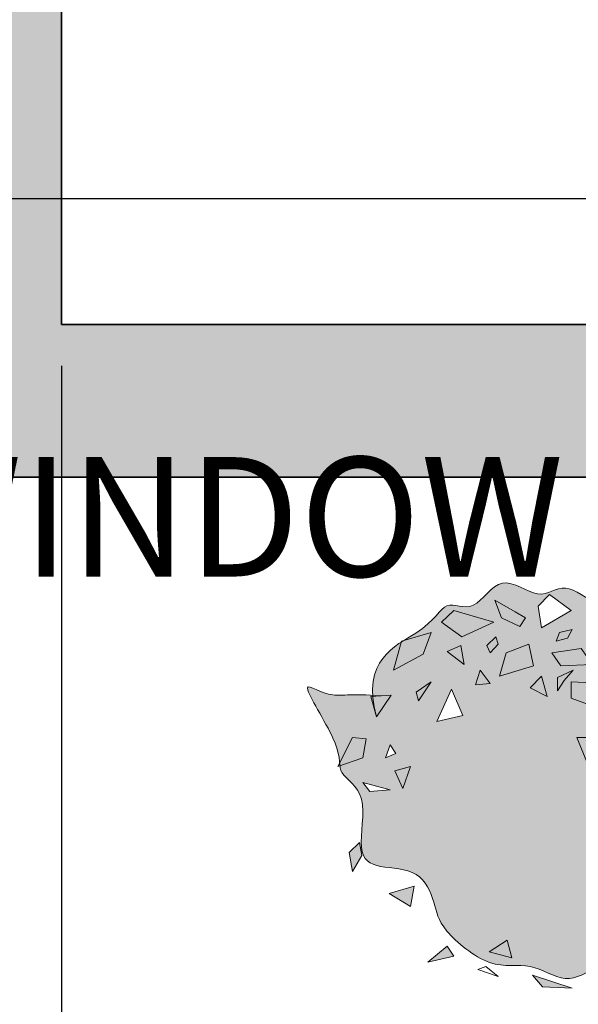
# Model space of a CAD drawing. Units: metres. Extents: x 4298.5 to 4325.2, y 2075 to 2095.8.
# Tile 5 of 35: x 4305.827 to 4306.669, y 2079.034 to 2080.517. Entities that reach past the tile are written whole.
import ezdxf

# ---------------------------------------------------------------- set-up
doc = ezdxf.new("R2010")
doc.units = ezdxf.units.M
for name, color, linetype, lineweight in [('A-ANNO-DIMS', 2, 'Continuous', 18), ('A-WALL', 7, 'Continuous', 35), ('A-WALL-PATT', 252, 'Continuous', 13), ('L-PLNT', 94, 'Continuous', 13)]:
    doc.layers.add(name, color=color, linetype=linetype, lineweight=lineweight)
doc.layers.add('L-PLNT-PATT', color=116, linetype='Continuous', lineweight=13, true_color=0x13823e)
doc.styles.get("Standard").update_dxf_attribs({"font": 'arial.ttf'})
doc.dimstyles.get("Standard").update_dxf_attribs({"dimtxt": 0.18, "dimasz": 0.18, "dimexe": 0.18, "dimexo": 0.0625, "dimgap": 0.09, "dimtad": 0, "dimtih": 1, "dimtoh": 1, "dimdec": 4, "dimzin": 0, "dimdsep": 46, "dimtxsty": 'Standard', "dimcen": 0.09, "dimadec": 0, "dimazin": 0, "dimtfac": 1, "dimtdec": 4, "dimtofl": 0, "dimtmove": 0, "dimatfit": 3, "dimfxl": 1, "dimtolj": 1, "dimtzin": 0, "dimarcsym": 0})

# ---------------------------------------------------------------- blocks, each defined once
blk = doc.blocks.new('*U9')
for points in [[(1.237, 12.003), (0.562, 11.31), (0.764, 10.013), (2.519, 11.051)], [(-2.003, 11.656), (-1.598, 10.618), (-0.518, 10.099), (-0.181, 10.618), (-0.788, 10.964)], [(4.139, 11.137), (3.599, 10.013), (4.004, 9.234), (5.218, 8.715), (6.298, 9.407), (5.083, 10.186), (4.611, 10.013)], [(-4.432, 11.051), (-5.175, 10.359), (-3.96, 9.493), (-2.07, 10.359)], [(-5.782, 9.753), (-7.537, 9.234), (-8.009, 7.504), (-6.255, 8.455)], [(-1.935, 9.493), (-2.475, 8.974), (-2.273, 8.542), (-1.8, 9.061)], [(2.586, 9.926), (1.844, 9.753), (1.642, 9.234), (2.316, 9.407)], [(-4.837, 8.628), (-3.825, 7.85), (-4.027, 8.974)], [(0.022, 9.061), (-1.328, 8.542), (-1.733, 7.157), (0.292, 7.763)], [(1.372, 8.542), (3.126, 8.801), (3.801, 7.85), (1.912, 7.763)], [(7.446, 9.32), (7.108, 7.936), (8.525, 7.936)], [(4.611, 8.282), (4.544, 7.763), (4.949, 7.59), (4.949, 8.282)], [(6.433, 7.936), (5.488, 7.676), (5.556, 6.206), (6.501, 6.638)], [(-2.88, 7.504), (-3.15, 6.638), (-2.273, 6.725)], [(0.764, 7.157), (0.089, 6.465), (1.102, 5.946)], [(1.709, 6.292), (1.709, 7.071), (2.654, 7.504), (2.114, 6.898)], [(-5.782, 6.811), (-6.659, 6.206), (-6.524, 5.687)], [(2.519, 6.811), (2.519, 5.86), (4.409, 5.167), (4.611, 6.725)], [(7.851, 6.811), (7.176, 6.206), (8.998, 5.514), (9.335, 6.379)], [(-8.144, 6.033), (-9.359, 5.946), (-9.022, 4.735)], [(-4.567, 6.379), (-5.445, 4.475), (-3.892, 4.821)], [(5.488, 5.514), (5.421, 4.821), (6.163, 5.081)], [(8.12, 4.994), (7.108, 4.648), (6.501, 4.129), (7.378, 3.091), (8.12, 3.524), (7.648, 3.87)], [(8.728, 4.735), (8.188, 4.562), (8.39, 3.87), (8.593, 4.043)], [(10.28, 5.167), (9.2, 4.043), (8.998, 2.312), (10.482, 0.495), (11.765, 0.409), (10.348, 2.485), (9.335, 2.399), (10.28, 2.831)], [(4.409, 4.562), (4.274, 3.697), (5.488, 3.264)], [(-11.316, 1.793), (-9.831, 2.312), (-9.629, 3.437), (-10.439, 3.524)], [(3.531, 1.88), (2.856, 3.524), (3.801, 3.524)], [(-8.212, 3.091), (-8.482, 2.312), (-7.874, 2.572)], [(4.274, 2.745), (5.286, 2.658), (4.409, 1.274)], [(8.188, 2.572), (7.918, 2.053), (8.66, 1.534)], [(-6.997, 1.793), (-7.942, 1.534), (-7.469, 0.495)], [(7.513, 1.707), (6.906, 1.274), (6.231, 2.139)], [(5.826, 1.534), (5.016, 0.409), (5.488, -0.024), (6.501, 0.409)], [(-8.212, 0.409), (-9.426, 0.322), (-9.831, 0.841)], [(8.12, 0.755), (7.513, 0.149), (8.93, -0.283), (9.133, 0.495)], [(7.783, -0.803), (6.433, -1.495), (6.433, -0.716)], [(10.078, -0.629), (9.74, -1.322), (10.482, -0.889)], [(8.323, -1.754), (7.985, -2.533), (7.581, -2.1)], [(9.335, -1.754), (9.538, -3.744), (10.145, -2.533)], [(-10.034, -2.706), (-10.641, -3.312), (-10.439, -4.436), (-9.899, -3.485)], [(9.335, -5.129), (8.458, -6.253), (7.985, -5.215)], [(-8.279, -5.734), (-6.794, -5.302), (-6.997, -6.513)], [(6.096, -8.935), (6.163, -7.205), (6.906, -6.686), (7.243, -7.378)], [(8.053, -8.07), (8.593, -7.118), (7.918, -7.551)], [(5.286, -7.984), (4.611, -8.157), (5.016, -8.935)], [(-2.34, -9.195), (-1.26, -8.503), (-0.99, -9.541)], [(-4.837, -8.849), (-4.432, -9.454), (-5.985, -9.801)], [(4.071, -9.454), (3.531, -9.974), (4.071, -10.579), (4.611, -9.887)], [(6.028, -9.454), (5.421, -9.974), (6.163, -10.147)], [(-2.543, -10.06), (-3.015, -10.233), (-1.8, -10.666)], [(0.224, -10.579), (0.832, -11.272), (2.586, -11.358)]]:
    blk.add_lwpolyline(points, close=True)
blk = doc.blocks.new('*D23')
at = {"layer": 'A-ANNO-DIMS', "color": 0, "lineweight": -2, "transparency": 16777216}
for p, q in [((4308.1606, 2079.8556), (4308.1606, 2079.5881)), ((4309.1606, 2079.8556), (4309.1606, 2079.5881)), ((4308.1606, 2079.7681), (4307.9806, 2079.7681)), ((4308.9806, 2079.7681), (4308.3406, 2079.7681))]:
    blk.add_line(p, q, dxfattribs=at)
at = {"layer": 'A-ANNO-DIMS', "color": 0, "transparency": 16777216}
for points in [[(4308.3406, 2079.7981), (4308.3406, 2079.7381), (4308.1606, 2079.7681)], [(4308.9806, 2079.7981), (4308.9806, 2079.7381), (4309.1606, 2079.7681)]]:
    blk.add_solid(points, dxfattribs=at)
at = {"layer": 'Defpoints', "color": 0, "transparency": 16777216}
for p in [(4308.1606, 2079.9181), (4309.1606, 2079.9181), (4308.1606, 2079.7681)]:
    blk.add_point(p, dxfattribs=at)
at = {"layer": 'A-ANNO-DIMS', "color": 0, "transparency": 16777216, "insert": (4306.7086, 2079.7681), "char_height": 0.18, "attachment_point": 5}
blk.add_mtext('\\A1;WINDOW W1 1 TYP.', dxfattribs=at)
blk = doc.blocks.new('*D47')
at = {"layer": 'A-ANNO-DIMS', "color": 0, "lineweight": -2, "transparency": 16777216}
for p, q in [((4300.4306, 2084.4956), (4300.4306, 2074.9896)), ((4322.8106, 2084.4956), (4322.8106, 2074.9896)), ((4300.6106, 2075.1696), (4311.2252, 2075.1696)), ((4322.6306, 2075.1696), (4312.016, 2075.1696))]:
    blk.add_line(p, q, dxfattribs=at)
at = {"layer": 'A-ANNO-DIMS', "color": 0, "transparency": 16777216}
for points in [[(4300.6106, 2075.1996), (4300.6106, 2075.1396), (4300.4306, 2075.1696)], [(4322.6306, 2075.1996), (4322.6306, 2075.1396), (4322.8106, 2075.1696)]]:
    blk.add_solid(points, dxfattribs=at)
at = {"layer": 'Defpoints', "color": 0, "transparency": 16777216}
for p in [(4300.4306, 2084.5581), (4322.8106, 2084.5581), (4322.8106, 2075.1696)]:
    blk.add_point(p, dxfattribs=at)
at = {"layer": 'A-ANNO-DIMS', "color": 0, "transparency": 16777216, "insert": (4311.6206, 2075.1696), "char_height": 0.18, "attachment_point": 5}
blk.add_mtext('\\A1;22.38', dxfattribs=at)
blk = doc.blocks.new('*D54')
at = {"layer": 'A-ANNO-DIMS', "color": 0, "lineweight": -2, "transparency": 16777216}
for p, q in [((4305.5981, 2079.8281), (4299.0921, 2079.8281)), ((4299.2721, 2079.6481), (4299.2721, 2078.26)), ((4299.2721, 2076.5081), (4299.2721, 2077.8961)), ((4309.0981, 2076.3281), (4299.0921, 2076.3281))]:
    blk.add_line(p, q, dxfattribs=at)
at = {"layer": 'A-ANNO-DIMS', "color": 0, "transparency": 16777216}
for points in [[(4299.2421, 2079.6481), (4299.3021, 2079.6481), (4299.2721, 2079.8281)], [(4299.2421, 2076.5081), (4299.3021, 2076.5081), (4299.2721, 2076.3281)]]:
    blk.add_solid(points, dxfattribs=at)
at = {"layer": 'Defpoints', "color": 0, "transparency": 16777216}
for p in [(4305.6606, 2079.8281), (4299.2721, 2076.3281), (4309.1606, 2076.3281)]:
    blk.add_point(p, dxfattribs=at)
at = {"layer": 'A-ANNO-DIMS', "color": 0, "transparency": 16777216, "insert": (4299.2721, 2078.0781), "char_height": 0.18, "attachment_point": 5}
blk.add_mtext('\\A1;3.5', dxfattribs=at)
blk = doc.blocks.new('*D59')
at = {"layer": 'A-ANNO-DIMS', "color": 0, "lineweight": -2, "transparency": 16777216}
for p, q in [((4305.8906, 2079.9956), (4305.8906, 2074.9896)), ((4307.3906, 2079.9956), (4307.3906, 2074.9896)), ((4306.0706, 2075.1696), (4306.3945, 2075.1696)), ((4307.2106, 2075.1696), (4306.8866, 2075.1696))]:
    blk.add_line(p, q, dxfattribs=at)
at = {"layer": 'A-ANNO-DIMS', "color": 0, "transparency": 16777216}
for points in [[(4306.0706, 2075.1996), (4306.0706, 2075.1396), (4305.8906, 2075.1696)], [(4307.2106, 2075.1996), (4307.2106, 2075.1396), (4307.3906, 2075.1696)]]:
    blk.add_solid(points, dxfattribs=at)
at = {"layer": 'Defpoints', "color": 0, "transparency": 16777216}
for p in [(4305.8906, 2080.0581), (4307.3906, 2080.0581), (4307.3906, 2075.1696)]:
    blk.add_point(p, dxfattribs=at)
at = {"layer": 'A-ANNO-DIMS', "color": 0, "transparency": 16777216, "insert": (4306.6406, 2075.1696), "char_height": 0.18, "attachment_point": 5}
blk.add_mtext('\\A1;1.5', dxfattribs=at)
blk = doc.blocks.new('*D60')
at = {"layer": 'A-ANNO-DIMS', "color": 0, "lineweight": -2, "transparency": 16777216}
for p, q in [((4305.9531, 2081.9381), (4324.7671, 2081.9381)), ((4324.5871, 2081.7581), (4324.5871, 2081.18)), ((4324.5871, 2080.2381), (4324.5871, 2080.8162)), ((4305.9531, 2080.0581), (4324.7671, 2080.0581))]:
    blk.add_line(p, q, dxfattribs=at)
at = {"layer": 'A-ANNO-DIMS', "color": 0, "transparency": 16777216}
for points in [[(4324.5571, 2081.7581), (4324.6171, 2081.7581), (4324.5871, 2081.9381)], [(4324.5571, 2080.2381), (4324.6171, 2080.2381), (4324.5871, 2080.0581)]]:
    blk.add_solid(points, dxfattribs=at)
at = {"layer": 'Defpoints', "color": 0, "transparency": 16777216}
for p in [(4305.8906, 2081.9381), (4324.5871, 2081.9381), (4305.8906, 2080.0581)]:
    blk.add_point(p, dxfattribs=at)
at = {"layer": 'A-ANNO-DIMS', "color": 0, "transparency": 16777216, "insert": (4324.5871, 2080.9981), "char_height": 0.18, "attachment_point": 5}
blk.add_mtext('\\A1;1.88', dxfattribs=at)
blk = doc.blocks.new('*D64')
at = {"layer": 'A-ANNO-DIMS', "color": 0, "lineweight": -2, "transparency": 16777216}
for p, q in [((4312.1097, 2081.1221), (4299.0921, 2081.1221)), ((4299.2721, 2080.9421), (4299.2721, 2080.427)), ((4312.1097, 2080.247), (4299.0921, 2080.247)), ((4299.2721, 2080.247), (4299.2721, 2080.067)), ((4299.2721, 2080.067), (4299.0921, 2080.067))]:
    blk.add_line(p, q, dxfattribs=at)
at = {"layer": 'A-ANNO-DIMS', "color": 0, "transparency": 16777216}
for points in [[(4299.2421, 2080.9421), (4299.3021, 2080.9421), (4299.2721, 2081.1221)], [(4299.2421, 2080.427), (4299.3021, 2080.427), (4299.2721, 2080.247)]]:
    blk.add_solid(points, dxfattribs=at)
at = {"layer": 'Defpoints', "color": 0, "transparency": 16777216}
for p in [(4312.1722, 2081.1221), (4299.2721, 2080.247), (4312.1722, 2080.247)]:
    blk.add_point(p, dxfattribs=at)
at = {"layer": 'A-ANNO-DIMS', "color": 0, "transparency": 16777216, "insert": (4298.7681, 2080.067), "char_height": 0.18, "attachment_point": 5}
blk.add_mtext('\\A1;0.88', dxfattribs=at)
blk = doc.blocks.new('*D78')
at = {"layer": 'A-ANNO-DIMS', "color": 0, "lineweight": -2, "transparency": 16777216}
for p, q in [((4312.4969, 2079.7393), (4312.4969, 2079.9193)), ((4312.4069, 2079.8293), (4312.5869, 2079.8293)), ((4305.3847, 2076.7806), (4307.8863, 2077.853)), ((4305.2047, 2076.7806), (4305.3847, 2076.7806))]:
    blk.add_line(p, q, dxfattribs=at)
at = {"layer": 'A-ANNO-DIMS', "color": 0, "transparency": 16777216}
blk.add_solid([(4307.8745, 2077.8806), (4307.8981, 2077.8254), (4308.0518, 2077.9239)], dxfattribs=at)
at = {"layer": 'Defpoints', "color": 0, "transparency": 16777216}
for p in [(4312.4969, 2079.8293), (4308.0518, 2077.9239)]:
    blk.add_point(p, dxfattribs=at)
at = {"layer": 'A-ANNO-DIMS', "color": 0, "transparency": 16777216, "insert": (4304.53, 2076.7806), "char_height": 0.18, "attachment_point": 5}
blk.add_mtext('\\A1;2X R4.836', dxfattribs=at)

msp = doc.modelspace()

# ---------------------------------------------------------------- hatches: boundary and pattern name
at = {"layer": 'A-WALL-PATT'}
h = msp.add_hatch(color=256, dxfattribs=at)
h.dxf.hatch_style = 1
h.paths.add_polyline_path([(4308.7606, 2094.4781), (4308.1606, 2094.4781), (4307.4606, 2094.4781), (4307.4606, 2094.2481), (4308.2706, 2094.2481), (4308.2706, 2094.1281), (4308.3906, 2094.1281), (4308.3906, 2094.2481), (4308.7606, 2094.2481)])
h.paths.add_polyline_path([(4310.1206, 2094.4781), (4309.5206, 2094.4781), (4309.5206, 2094.2481), (4309.8906, 2094.2481), (4309.8906, 2092.2481), (4308.3906, 2092.2481), (4308.3906, 2093.4281), (4308.2706, 2093.4281), (4308.2706, 2092.0181), (4309.8906, 2092.0181), (4309.8906, 2087.0181), (4309.7706, 2087.0181), (4309.7706, 2086.7881), (4309.8906, 2086.7881), (4311.9406, 2086.7881), (4311.9406, 2087.0181), (4310.1206, 2087.0181), (4310.1206, 2089.0181), (4310.2406, 2089.0181), (4310.2406, 2089.1381), (4310.1206, 2089.1381), (4310.1206, 2092.0181), (4310.3078, 2092.0181), (4310.3078, 2092.2481), (4310.1206, 2092.2481)])
h.paths.add_polyline_path([(4311.7406, 2092.2481), (4311.0678, 2092.2481), (4311.0678, 2092.0181), (4311.7406, 2092.0181)], flags=17)
h.paths.add_polyline_path([(4313.1733, 2092.2481), (4312.5006, 2092.2481), (4312.5006, 2092.0181), (4313.1733, 2092.0181)])
h.paths.add_polyline_path([(4314.5378, 2092.2481), (4314.1206, 2092.2481), (4313.9333, 2092.2481), (4313.9333, 2092.0181), (4314.1206, 2092.0181), (4314.1206, 2087.0181), (4314.0006, 2087.0181), (4314.0006, 2086.7881), (4314.1206, 2086.7881), (4315.5718, 2086.7881), (4315.5718, 2087.0181), (4314.3506, 2087.0181), (4314.3506, 2092.0181), (4314.5378, 2092.0181)])
h.paths.add_polyline_path([(4315.9706, 2092.2481), (4315.2978, 2092.2481), (4315.2978, 2092.0181), (4315.9706, 2092.0181)])
h.paths.add_polyline_path([(4317.4033, 2092.2481), (4316.7306, 2092.2481), (4316.7306, 2092.0181), (4317.4033, 2092.0181)])
h.paths.add_polyline_path([(4318.9506, 2092.2481), (4318.3506, 2092.2481), (4318.1633, 2092.2481), (4318.1633, 2092.0181), (4318.3506, 2092.0181), (4318.3506, 2091.8981), (4318.5806, 2091.8981), (4318.5806, 2092.0181), (4318.9506, 2092.0181)])
h.paths.add_polyline_path([(4321.0106, 2092.2481), (4319.7106, 2092.2481), (4319.7106, 2092.0181), (4320.0806, 2092.0181), (4320.0806, 2090.0181), (4318.5806, 2090.0181), (4318.5806, 2091.1981), (4318.3506, 2091.1981), (4318.3506, 2090.0181), (4318.3506, 2087.0181), (4318.2306, 2087.0181), (4318.2306, 2086.7881), (4318.3506, 2086.7881), (4318.3506, 2086.3081), (4318.5806, 2086.3081), (4318.5806, 2089.7881), (4321.7806, 2089.7881), (4321.7806, 2090.0181), (4320.2006, 2090.0181), (4320.2006, 2092.0181), (4321.0106, 2092.0181)])
h.paths.add_polyline_path([(4322.8106, 2092.2481), (4321.7706, 2092.2481), (4321.7706, 2092.0181), (4322.5806, 2092.0181), (4322.5806, 2091.2831), (4322.8106, 2091.2831)])
h.paths.add_polyline_path([(4322.8106, 2090.5231), (4322.5806, 2090.5231), (4322.5806, 2089.7881), (4322.5806, 2089.5254), (4322.8106, 2089.5254), (4322.8106, 2090.0181)])
h.paths.add_polyline_path([(4322.8106, 2088.7654), (4322.5806, 2088.7654), (4322.5806, 2087.6681), (4322.8106, 2087.6681)])
h.paths.add_polyline_path([(4322.8106, 2086.9081), (4322.5806, 2086.9081), (4322.5806, 2085.8107), (4322.8106, 2085.8107)])
h.paths.add_polyline_path([(4322.8106, 2085.0507), (4322.5806, 2085.0507), (4322.5806, 2084.7881), (4318.5806, 2084.7881), (4318.5806, 2085.0581), (4318.5806, 2085.4081), (4318.3506, 2085.4081), (4318.3506, 2084.5581), (4318.3506, 2080.8581), (4318.4706, 2080.8581), (4318.4706, 2082.3281), (4319.2606, 2082.3281), (4319.2606, 2082.5581), (4318.5806, 2082.5581), (4318.5806, 2084.5581), (4320.0806, 2084.5581), (4320.0806, 2083.9381), (4320.3106, 2083.9381), (4320.3106, 2084.5581), (4322.8106, 2084.5581)])
h.paths.add_polyline_path([(4320.3106, 2083.1781), (4320.0806, 2083.1781), (4320.0806, 2082.5581), (4319.9606, 2082.5581), (4319.9606, 2082.3281), (4320.0806, 2082.3281), (4320.0806, 2081.5731), (4320.3106, 2081.5731)], flags=17)
h.paths.add_polyline_path([(4320.3106, 2080.8131), (4320.0806, 2080.8131), (4320.0806, 2080.0581), (4318.4286, 2080.0581), (4318.4286, 2079.8281), (4320.3106, 2079.8281)])
h.paths.add_polyline_path([(4317.3506, 2085.2881), (4316.5718, 2085.2881), (4316.5718, 2085.0581), (4317.3506, 2085.0581)])
h.paths.add_polyline_path([(4315.5718, 2085.2881), (4314.8434, 2085.2881), (4314.8434, 2085.0581), (4315.5718, 2085.0581)])
h.paths.add_polyline_path([(4313.8434, 2085.2881), (4312.9406, 2085.2881), (4312.9406, 2085.0581), (4313.8434, 2085.0581)])
h.paths.add_polyline_path([(4311.9406, 2085.2881), (4311.4406, 2085.2881), (4311.4406, 2085.0581), (4311.9406, 2085.0581)])
h.paths.add_polyline_path([(4317.3306, 2087.0181), (4316.5718, 2087.0181), (4316.5718, 2086.7881), (4317.3306, 2086.7881)])
h.paths.add_polyline_path([(4313.1006, 2089.1381), (4311.1406, 2089.1381), (4311.1406, 2089.0181), (4312.9806, 2089.0181), (4312.9806, 2087.0181), (4312.9406, 2087.0181), (4312.9406, 2086.7881), (4313.1006, 2086.7881), (4313.1006, 2087.0181)])
h.paths.add_polyline_path([(4307.5515, 2087.0181), (4305.8906, 2087.0181), (4305.8906, 2092.2481), (4305.8906, 2094.2481), (4306.7006, 2094.2481), (4306.7006, 2094.4781), (4305.6606, 2094.4781), (4305.6606, 2092.2481), (4305.2906, 2092.2481), (4305.2906, 2092.0181), (4305.6606, 2092.0181), (4305.6606, 2090.0181), (4304.1606, 2090.0181), (4304.1606, 2091.1981), (4304.0406, 2091.1981), (4304.0406, 2089.9081), (4301.5606, 2089.9081), (4301.5606, 2089.7881), (4304.0406, 2089.7881), (4305.6606, 2089.7881), (4305.6606, 2086.6381), (4305.8906, 2086.6381), (4305.8906, 2086.7881), (4307.5515, 2086.7881)])
h.paths.add_polyline_path([(4307.5515, 2085.2881), (4305.8906, 2085.2881), (4305.8906, 2085.4381), (4305.6606, 2085.4381), (4305.6606, 2084.7881), (4305.2906, 2084.7881), (4305.2906, 2084.5581), (4305.6606, 2084.5581), (4305.6606, 2084.02), (4305.8906, 2084.02), (4305.8906, 2084.5581), (4305.8906, 2085.0581), (4307.5515, 2085.0581)])
h.paths.add_polyline_path([(4310.2406, 2085.2881), (4308.5515, 2085.2881), (4308.5515, 2085.0581), (4310.2406, 2085.0581)])
h.paths.add_polyline_path([(4317.4286, 2080.0581), (4316.5718, 2080.0581), (4316.5718, 2079.8281), (4317.4286, 2079.8281)])
h.paths.add_polyline_path([(4315.5718, 2080.0581), (4314.8434, 2080.0581), (4314.8434, 2079.8281), (4315.5718, 2079.8281)])
h.paths.add_polyline_path([(4313.8434, 2080.0581), (4312.9406, 2080.0581), (4312.9406, 2079.8281), (4313.8434, 2079.8281)])
h.paths.add_polyline_path([(4311.9406, 2080.0581), (4311.4406, 2080.0581), (4311.4406, 2079.8281), (4311.9406, 2079.8281)])
h.paths.add_polyline_path([(4310.2406, 2080.0581), (4310.1206, 2080.0581), (4310.1206, 2084.0381), (4309.8906, 2084.0381), (4309.8906, 2080.0581), (4309.1606, 2080.0581), (4309.1606, 2079.8281), (4310.2406, 2079.8281)])
h.paths.add_polyline_path([(4308.1606, 2080.0581), (4307.5106, 2080.0581), (4307.5106, 2080.1781), (4307.3906, 2080.1781), (4307.3906, 2080.0581), (4305.8906, 2080.0581), (4305.8906, 2080.567), (4305.6606, 2080.567), (4305.6606, 2079.8281), (4308.1606, 2079.8281)])
h.paths.add_polyline_path([(4307.5106, 2081.9381), (4309.0906, 2081.9381), (4309.0906, 2082.0581), (4305.8906, 2082.0581), (4305.8906, 2083.26), (4305.6606, 2083.26), (4305.6606, 2081.327), (4305.8906, 2081.327), (4305.8906, 2081.9381), (4307.3906, 2081.9381), (4307.3906, 2080.8781), (4307.5106, 2080.8781)])
h.paths.add_polyline_path([(4304.5306, 2084.7881), (4302.7306, 2084.7881), (4302.7306, 2084.5581), (4304.5306, 2084.5581)])
h.paths.add_polyline_path([(4301.9706, 2084.7881), (4300.6606, 2084.7881), (4300.6606, 2085.0249), (4300.4306, 2085.0249), (4300.4306, 2084.5581), (4301.9706, 2084.5581)])
h.paths.add_polyline_path([(4300.6606, 2086.8843), (4300.4306, 2086.8843), (4300.4306, 2085.7849), (4300.6606, 2085.7849)])
h.paths.add_polyline_path([(4300.6606, 2089.1618), (4300.4306, 2089.1618), (4300.4306, 2087.6443), (4300.6606, 2087.6443)])
h.paths.add_polyline_path([(4300.6606, 2091.0212), (4300.4306, 2091.0212), (4300.4306, 2089.9218), (4300.6606, 2089.9218)])
h.paths.add_polyline_path([(4300.6606, 2092.0181), (4301.9706, 2092.0181), (4301.9706, 2092.2481), (4300.4306, 2092.2481), (4300.4306, 2091.7812), (4300.6606, 2091.7812)])
h.paths.add_polyline_path([(4304.5306, 2092.2481), (4302.7306, 2092.2481), (4302.7306, 2092.0181), (4304.0406, 2092.0181), (4304.0406, 2091.8981), (4304.1606, 2091.8981), (4304.1606, 2092.0181), (4304.5306, 2092.0181)], flags=17)
at = {"layer": 'L-PLNT-PATT'}
h = msp.add_hatch(color=256, dxfattribs=at)
h.dxf.hatch_style = 1
edge = h.paths.add_edge_path()
edge.add_spline(control_points=[(4306.6904, 2079.0858), (4306.693, 2079.0871), (4306.7116, 2079.0964), (4306.7474, 2079.1062), (4306.802, 2079.1294), (4306.8313, 2079.1371), (4306.8126, 2079.1655), (4306.8652, 2079.1897), (4306.8314, 2079.216), (4306.8585, 2079.2758), (4306.8772, 2079.2952), (4306.8606, 2079.3237), (4306.9348, 2079.3686), (4306.8649, 2079.3982), (4306.8975, 2079.4058), (4306.8936, 2079.4409), (4306.8554, 2079.4776), (4306.874, 2079.4969), (4306.821, 2079.5479), (4306.821, 2079.5939), (4306.7731, 2079.5973), (4306.7527, 2079.6292), (4306.6995, 2079.6292), (4306.6471, 2079.6745), (4306.6123, 2079.6374), (4306.5517, 2079.6883), (4306.5118, 2079.6182), (4306.4672, 2079.6482), (4306.4529, 2079.6088), (4306.4126, 2079.5858), (4306.4062, 2079.5818)], knot_values=[0.818571, 0.818571, 0.818571, 0.818571, 0.97924, 1.97924, 2.97924, 3.97924, 4.97924, 5.97924, 6.97924, 7.97924, 8.97924, 9.97924, 10.97924, 11.97924, 12.97924, 13.97924, 14.97924, 15.97924, 16.97924, 17.97924, 18.97924, 19.97924, 20.97924, 21.97924, 22.97924, 23.97924, 24.97924, 25.97924, 26.97924, 27.16067, 27.16067, 27.16067, 27.16067], degree=3, periodic=0)
edge.add_line((4306.4062, 2079.5818), (4306.4475, 2079.594))
edge.add_line((4306.4475, 2079.594), (4306.4355, 2079.5611))
edge.add_line((4306.4355, 2079.5611), (4306.3909, 2079.5369))
edge.add_line((4306.3909, 2079.5369), (4306.4025, 2079.5795))
edge.add_spline(control_points=[(4306.4025, 2079.5795), (4306.3799, 2079.5648), (4306.3566, 2079.5439), (4306.3593, 2079.4995)], knot_values=[0.141368, 0.141368, 0.141368, 0.141368, 0.783694, 0.783694, 0.783694, 0.783694], degree=3, periodic=0)
edge.add_spline(control_points=[(4306.3593, 2079.4995), (4306.3633, 2079.4992), (4306.3675, 2079.4989), (4306.372, 2079.4984)], knot_values=[40.901028, 40.901028, 40.901028, 40.901028, 41, 41, 41, 41], degree=3, periodic=0)
edge.add_line((4306.372, 2079.4984), (4306.3875, 2079.4995))
edge.add_line((4306.3875, 2079.4995), (4306.3652, 2079.4666))
edge.add_line((4306.3652, 2079.4666), (4306.3566, 2079.4973))
edge.add_line((4306.3566, 2079.4973), (4306.3594, 2079.4975))
edge.add_spline(control_points=[(4306.3595, 2079.4975), (4306.3594, 2079.4982), (4306.3594, 2079.4988), (4306.3593, 2079.4995)], knot_values=[0.13204, 0.13204, 0.13204, 0.13204, 0.141368, 0.141368, 0.141368, 0.141368], degree=3, periodic=0)
edge.add_spline(control_points=[(4306.3593, 2079.4995), (4306.3231, 2079.5018), (4306.2915, 2079.492), (4306.2395, 2079.534), (4306.3065, 2079.4314), (4306.3089, 2079.4046), (4306.3096, 2079.3971)], knot_values=[37.439141, 37.439141, 37.439141, 37.439141, 38.340169, 39.340169, 40.340169, 40.901028, 40.901028, 40.901028, 40.901028], degree=3, periodic=0)
edge.add_line((4306.3096, 2079.3971), (4306.3292, 2079.4358))
edge.add_line((4306.3292, 2079.4358), (4306.3498, 2079.4336))
edge.add_line((4306.3498, 2079.4336), (4306.3446, 2079.405))
edge.add_line((4306.3446, 2079.405), (4306.31, 2079.3929))
edge.add_spline(control_points=[(4306.31, 2079.3929), (4306.3105, 2079.389), (4306.3136, 2079.3754), (4306.3549, 2079.3545), (4306.3335, 2079.2572), (4306.3657, 2079.2384), (4306.4319, 2079.2384), (4306.4547, 2079.1846), (4306.4582, 2079.1492), (4306.5392, 2079.0831), (4306.5975, 2079.0999), (4306.6479, 2079.063), (4306.677, 2079.0789), (4306.6904, 2079.0858)], knot_values=[27.16067, 27.16067, 27.16067, 27.16067, 27.490087, 28.490087, 29.490087, 30.490087, 31.490087, 32.490087, 33.490087, 34.490087, 35.490087, 36.490087, 37.329418, 37.329418, 37.329418, 37.329418], degree=3, periodic=0)
edge.add_line((4306.6904, 2079.0858), (4306.684, 2079.093))
edge.add_line((4306.684, 2079.093), (4306.6977, 2079.1062))
edge.add_line((4306.6977, 2079.1062), (4306.7115, 2079.0952))
h.paths.add_polyline_path([(4306.6669, 2079.4358), (4306.6909, 2079.4358), (4306.684, 2079.3941)], flags=16)
h.paths.add_polyline_path([(4306.7029, 2079.416), (4306.7286, 2079.4138), (4306.7063, 2079.3787)], flags=16)
h.paths.add_polyline_path([(4306.4955, 2079.4688), (4306.456, 2079.46), (4306.4783, 2079.5083)], flags=16)
h.paths.add_polyline_path([(4306.6223, 2079.4973), (4306.5966, 2079.5105), (4306.6137, 2079.5281)], flags=16)
h.paths.add_polyline_path([(4306.7029, 2079.4402), (4306.7063, 2079.4622), (4306.7337, 2079.4292)], flags=16)
h.paths.add_polyline_path([(4306.7217, 2079.3567), (4306.7423, 2079.3853), (4306.7595, 2079.3567), (4306.7337, 2079.3457)], flags=16)
h.paths.add_polyline_path([(4306.6583, 2079.4952), (4306.6583, 2079.5193), (4306.7115, 2079.5171), (4306.7063, 2079.4776)], flags=16)
h.paths.add_polyline_path([(4306.6377, 2079.5061), (4306.6377, 2079.5259), (4306.6617, 2079.5369), (4306.648, 2079.5215)], flags=16)
h.paths.add_polyline_path([(4306.5366, 2079.5171), (4306.5143, 2079.5149), (4306.5212, 2079.5369)], flags=16)
h.paths.add_polyline_path([(4306.5503, 2079.5281), (4306.5606, 2079.5633), (4306.5949, 2079.5765), (4306.6018, 2079.5435)], flags=16)
h.paths.add_polyline_path([(4306.4166, 2079.3919), (4306.4046, 2079.3589), (4306.3926, 2079.3853)], flags=16)
h.paths.add_polyline_path([(4306.7526, 2079.4006), (4306.7852, 2079.3897), (4306.7697, 2079.3787)], flags=16)
h.paths.add_polyline_path([(4306.732, 2079.4688), (4306.7337, 2079.4864), (4306.7509, 2079.4754)], flags=16)
h.paths.add_polyline_path([(4306.6429, 2079.5435), (4306.6292, 2079.5633), (4306.6737, 2079.5699), (4306.6909, 2079.5457)], flags=16)
h.paths.add_polyline_path([(4306.7577, 2079.3281), (4306.792, 2079.3259), (4306.7577, 2079.3083)], flags=16)
h.paths.add_polyline_path([(4306.3943, 2079.4116), (4306.3789, 2079.405), (4306.3858, 2079.4248)], flags=16)
h.paths.add_polyline_path([(4306.4972, 2079.5457), (4306.4715, 2079.5655), (4306.4921, 2079.5743)], flags=16)
h.paths.add_polyline_path([(4306.4286, 2079.4908), (4306.4252, 2079.5039), (4306.4475, 2079.5193)], flags=16)
h.paths.add_polyline_path([(4306.5366, 2079.5633), (4306.5315, 2079.5743), (4306.5452, 2079.5874), (4306.5486, 2079.5765)], flags=16)
h.paths.add_polyline_path([(4306.7595, 2079.4512), (4306.7749, 2079.4644), (4306.8006, 2079.4732), (4306.7886, 2079.4446), (4306.8006, 2079.4358), (4306.7817, 2079.4248)], flags=16)
h.paths.add_polyline_path([(4306.3858, 2079.3567), (4306.3549, 2079.3545), (4306.3446, 2079.3677)], flags=16)
h.paths.add_polyline_path([(4306.7355, 2079.5039), (4306.7337, 2079.5413), (4306.7577, 2079.5479), (4306.7595, 2079.5149)], flags=16)
h.paths.add_polyline_path([(4306.7852, 2079.3501), (4306.8006, 2079.3655), (4306.8263, 2079.3589), (4306.8212, 2079.3391)], flags=16)
h.paths.add_polyline_path([(4306.7098, 2079.5435), (4306.7115, 2079.5567), (4306.72, 2079.5567), (4306.72, 2079.5391)], flags=16)
h.paths.add_polyline_path([(4306.636, 2079.5809), (4306.6412, 2079.594), (4306.66, 2079.5984), (4306.6532, 2079.5852)], flags=16)
h.paths.add_polyline_path([(4306.7955, 2079.3985), (4306.8023, 2079.4116), (4306.8143, 2079.3853)], flags=16)
h.paths.add_polyline_path([(4306.7869, 2079.293), (4306.8057, 2079.3018), (4306.7972, 2079.282)], flags=16)
h.paths.add_polyline_path([(4306.5812, 2079.6028), (4306.5537, 2079.616), (4306.5435, 2079.6424), (4306.5743, 2079.6248), (4306.5897, 2079.616)], flags=16)
h.paths.add_polyline_path([(4306.6137, 2079.6006), (4306.6086, 2079.6336), (4306.6258, 2079.6512), (4306.6583, 2079.627)], flags=16)
h.paths.add_polyline_path([(4306.4938, 2079.5874), (4306.4629, 2079.6094), (4306.4818, 2079.627), (4306.5418, 2079.6094)], flags=16)
h.paths.add_polyline_path([(4306.7766, 2079.5039), (4306.7938, 2079.5193), (4306.8314, 2079.5083), (4306.8229, 2079.4864)], flags=16)
h.paths.add_polyline_path([(4306.696, 2079.5809), (4306.6858, 2079.6006), (4306.6995, 2079.6292), (4306.7115, 2079.6006), (4306.7234, 2079.605), (4306.7543, 2079.5852), (4306.7269, 2079.5677)], flags=16)
h.paths.add_polyline_path([(4306.8074, 2079.4446), (4306.8023, 2079.4622), (4306.816, 2079.4666), (4306.8126, 2079.449)], flags=16)
h.paths.add_polyline_path([(4306.8229, 2079.405), (4306.828, 2079.449), (4306.8554, 2079.4776), (4306.8554, 2079.4182), (4306.8314, 2079.4072), (4306.8572, 2079.4094), (4306.8932, 2079.3567), (4306.8606, 2079.3589)], flags=16)
h.paths.add_polyline_path([(4306.5623, 2079.1303), (4306.5692, 2079.104), (4306.5349, 2079.1128)], flags=16)
h.paths.add_polyline_path([(4306.7749, 2079.5479), (4306.7835, 2079.583), (4306.8109, 2079.5479)], flags=16)
h.paths.add_polyline_path([(4306.8314, 2079.3018), (4306.852, 2079.282), (4306.8366, 2079.2512)], flags=16)
h.paths.add_polyline_path([(4306.8417, 2079.3127), (4306.8503, 2079.3303), (4306.8606, 2079.3237)], flags=16)
h.paths.add_polyline_path([(4306.7115, 2079.1391), (4306.7286, 2079.1435), (4306.7217, 2079.1194)], flags=16)
h.paths.add_polyline_path([(4306.7972, 2079.2139), (4306.8314, 2079.216), (4306.8092, 2079.1875)], flags=16)
h.paths.add_polyline_path([(4306.7509, 2079.1633), (4306.7697, 2079.1765), (4306.7783, 2079.1589), (4306.7492, 2079.1194)], flags=16)
h.paths.add_polyline_path([(4306.7955, 2079.1545), (4306.8126, 2079.1655), (4306.7989, 2079.1413)], flags=16)
h = msp.add_hatch(color=256, dxfattribs=at)
h.dxf.hatch_style = 1
h.paths.add_polyline_path([(4306.7063, 2079.4776), (4306.7115, 2079.5171), (4306.6583, 2079.5193), (4306.6583, 2079.4952)])
h.paths.add_polyline_path([(4306.7526, 2079.4006), (4306.7697, 2079.3787), (4306.7852, 2079.3897)])
h.paths.add_polyline_path([(4306.7337, 2079.5413), (4306.7355, 2079.5039), (4306.7595, 2079.5149), (4306.7577, 2079.5479)])
h.paths.add_polyline_path([(4306.7543, 2079.5852), (4306.7234, 2079.605), (4306.7115, 2079.6006), (4306.6995, 2079.6292), (4306.6858, 2079.6006), (4306.696, 2079.5809), (4306.7269, 2079.5677)])
h.paths.add_polyline_path([(4306.6, 2079.0776), (4306.6155, 2079.06), (4306.66, 2079.0578)])
h.paths.add_polyline_path([(4306.5812, 2079.6028), (4306.5897, 2079.616), (4306.5743, 2079.6248), (4306.5435, 2079.6424), (4306.5537, 2079.616)])
h.paths.add_polyline_path([(4306.4818, 2079.627), (4306.4629, 2079.6094), (4306.4938, 2079.5874), (4306.5418, 2079.6094)])
h.paths.add_polyline_path([(4306.5606, 2079.5633), (4306.5503, 2079.5281), (4306.6018, 2079.5435), (4306.5949, 2079.5765)])
h.paths.add_polyline_path([(4306.5486, 2079.5765), (4306.5452, 2079.5874), (4306.5315, 2079.5743), (4306.5366, 2079.5633)])
h.paths.add_polyline_path([(4306.5212, 2079.5369), (4306.5143, 2079.5149), (4306.5366, 2079.5171)])
h.paths.add_polyline_path([(4306.4972, 2079.5457), (4306.4921, 2079.5743), (4306.4715, 2079.5655)])
h.paths.add_polyline_path([(4306.4029, 2079.5809), (4306.3909, 2079.5369), (4306.4355, 2079.5611), (4306.4475, 2079.594)])
h.paths.add_polyline_path([(4306.4475, 2079.5193), (4306.4252, 2079.5039), (4306.4286, 2079.4908)])
h.paths.add_polyline_path([(4306.3566, 2079.4973), (4306.3652, 2079.4666), (4306.3875, 2079.4995)])
h.paths.add_polyline_path([(4306.3069, 2079.3919), (4306.3446, 2079.405), (4306.3498, 2079.4336), (4306.3292, 2079.4358)])
h.paths.add_polyline_path([(4306.4166, 2079.3919), (4306.3926, 2079.3853), (4306.4046, 2079.3589)])
h.paths.add_polyline_path([(4306.3429, 2079.2578), (4306.3395, 2079.2776), (4306.3241, 2079.2622), (4306.3292, 2079.2336)])
h.paths.add_polyline_path([(4306.4218, 2079.2116), (4306.3841, 2079.2007), (4306.4166, 2079.1809)])
h.paths.add_polyline_path([(4306.4423, 2079.0974), (4306.4818, 2079.1062), (4306.4715, 2079.1215)])
h.paths.add_polyline_path([(4306.5623, 2079.1303), (4306.5349, 2079.1128), (4306.5692, 2079.104)])
h.paths.add_polyline_path([(4306.6977, 2079.1062), (4306.684, 2079.093), (4306.6977, 2079.0776), (4306.7115, 2079.0952)])
h.paths.add_polyline_path([(4306.7783, 2079.1589), (4306.7697, 2079.1765), (4306.7509, 2079.1633), (4306.7492, 2079.1194)])
h.paths.add_polyline_path([(4306.7474, 2079.1062), (4306.732, 2079.093), (4306.7509, 2079.0886)])
h.paths.add_polyline_path([(4306.7955, 2079.1545), (4306.7989, 2079.1413), (4306.8126, 2079.1655)])
h.paths.add_polyline_path([(4306.8366, 2079.2512), (4306.852, 2079.282), (4306.8314, 2079.3018)])
h.paths.add_polyline_path([(4306.7217, 2079.3567), (4306.7337, 2079.3457), (4306.7595, 2079.3567), (4306.7423, 2079.3853)])
h.paths.add_polyline_path([(4306.8606, 2079.3589), (4306.8932, 2079.3567), (4306.8572, 2079.4094), (4306.8314, 2079.4072), (4306.8554, 2079.4182), (4306.8554, 2079.4776), (4306.828, 2079.449), (4306.8229, 2079.405)])
h.paths.add_polyline_path([(4306.8006, 2079.3655), (4306.7852, 2079.3501), (4306.8212, 2079.3391), (4306.8263, 2079.3589)])
h.paths.add_polyline_path([(4306.8606, 2079.3237), (4306.8503, 2079.3303), (4306.8417, 2079.3127)])
h.paths.add_polyline_path([(4306.8006, 2079.4732), (4306.7749, 2079.4644), (4306.7595, 2079.4512), (4306.7817, 2079.4248), (4306.8006, 2079.4358), (4306.7886, 2079.4446)])
h.paths.add_polyline_path([(4306.8023, 2079.4622), (4306.8074, 2079.4446), (4306.8126, 2079.449), (4306.816, 2079.4666)])
h.paths.add_polyline_path([(4306.8229, 2079.4864), (4306.8314, 2079.5083), (4306.7938, 2079.5193), (4306.7766, 2079.5039)])
h.paths.add_polyline_path([(4306.7337, 2079.4292), (4306.7063, 2079.4622), (4306.7029, 2079.4402)])
h.paths.add_polyline_path([(4306.6909, 2079.4358), (4306.6669, 2079.4358), (4306.684, 2079.3941)])
h.paths.add_polyline_path([(4306.7286, 2079.4138), (4306.7029, 2079.416), (4306.7063, 2079.3787)])
h.paths.add_polyline_path([(4306.6909, 2079.5457), (4306.6737, 2079.5699), (4306.6292, 2079.5633), (4306.6429, 2079.5435)])
h.paths.add_polyline_path([(4306.648, 2079.5215), (4306.6617, 2079.5369), (4306.6377, 2079.5259), (4306.6377, 2079.5061)])
h.paths.add_polyline_path([(4306.6137, 2079.5281), (4306.5966, 2079.5105), (4306.6223, 2079.4973)])
h.paths.add_polyline_path([(4306.6532, 2079.5852), (4306.66, 2079.5984), (4306.6412, 2079.594), (4306.636, 2079.5809)])
h.paths.add_polyline_path([(4306.7835, 2079.583), (4306.7749, 2079.5479), (4306.8109, 2079.5479)])

# ---------------------------------------------------------------- linework, layer by layer
at = {"layer": 'A-WALL'}
for p, q in [((4305.8906, 2081.9381), (4305.8906, 2080.0581)), ((4305.8906, 2080.0581), (4307.3906, 2080.0581)), ((4310.2406, 2079.8281), (4305.6606, 2079.8281))]:
    msp.add_line(p, q, dxfattribs=at)
at = {"layer": 'L-PLNT'}
msp.add_open_spline([(4306.3652, 2079.4666), (4306.3411, 2079.5531), (4306.4475, 2079.594), (4306.4672, 2079.6482), (4306.5118, 2079.6182), (4306.5517, 2079.6883), (4306.6123, 2079.6374), (4306.6471, 2079.6745), (4306.6995, 2079.6292), (4306.7527, 2079.6292), (4306.7731, 2079.5973), (4306.821, 2079.5939), (4306.821, 2079.5479), (4306.874, 2079.4969), (4306.8554, 2079.4776), (4306.8936, 2079.4409), (4306.8975, 2079.4058), (4306.8649, 2079.3982), (4306.9348, 2079.3686), (4306.8606, 2079.3237), (4306.8772, 2079.2952), (4306.8585, 2079.2758), (4306.8314, 2079.216), (4306.8652, 2079.1897), (4306.8126, 2079.1655), (4306.8313, 2079.1371), (4306.802, 2079.1294), (4306.7474, 2079.1062), (4306.6977, 2079.0926), (4306.6507, 2079.0609), (4306.5975, 2079.0999), (4306.5392, 2079.0831), (4306.4582, 2079.1492), (4306.4547, 2079.1846), (4306.4319, 2079.2384), (4306.3657, 2079.2384), (4306.3335, 2079.2572), (4306.3549, 2079.3545), (4306.3017, 2079.3815), (4306.318, 2079.4138), (4306.2395, 2079.534), (4306.2933, 2079.4906), (4306.3264, 2079.503), (4306.372, 2079.4984)], degree=3, dxfattribs=at)

# ---------------------------------------------------------------- block references
at = {"layer": 'L-PLNT', "xscale": 0.0254, "yscale": 0.0254, "zscale": 0.0254}
msp.add_blockref('*U9', (4306.5943, 2079.3463), dxfattribs=at)

# ---------------------------------------------------------------- dimensions: what is measured, and where the dimension line sits
at = {"layer": 'A-ANNO-DIMS'}
for base, p1, p2, override, picture, middle in [((4322.8106, 2075.1696), (4300.4306, 2084.5581), (4322.8106, 2084.5581), {"dimdec": 2, "dimlfac": 1, "dimrnd": 0, "dimzin": 0, "dimdsep": 46, "dimlunit": 2}, '*D47', (4311.6206, 2075.1696)), ((4307.3906, 2075.1696), (4305.8906, 2080.0581), (4307.3906, 2080.0581), {"dimdec": 1, "dimlfac": 1, "dimrnd": 0, "dimzin": 0, "dimdsep": 46, "dimlunit": 2}, '*D59', (4306.6406, 2075.1696))]:
    dim = msp.add_linear_dim(base=base, p1=p1, p2=p2, dimstyle='Standard', override=override, dxfattribs=at)
    dim.commit()
    dim.dimension.update_dxf_attribs({"geometry": picture, "text_midpoint": middle})
for base, p1, p2, override, picture, middle in [((4324.5871, 2081.9381), (4305.8906, 2080.0581), (4305.8906, 2081.9381), {"dimdec": 2, "dimlfac": 1, "dimrnd": 0, "dimzin": 0, "dimdsep": 46, "dimlunit": 2}, '*D60', (4324.5871, 2080.9981)), ((4299.2721, 2080.247), (4312.1722, 2081.1221), (4312.1722, 2080.247), {"dimdec": 2, "dimlfac": 1, "dimrnd": 0, "dimzin": 0, "dimdsep": 46, "dimlunit": 2}, '*D64', (4298.7681, 2080.067)), ((4299.2721, 2076.3281), (4305.6606, 2079.8281), (4309.1606, 2076.3281), {"dimdec": 1, "dimlfac": 1, "dimrnd": 0, "dimzin": 0, "dimdsep": 46, "dimlunit": 2}, '*D54', (4299.2721, 2078.0781))]:
    dim = msp.add_linear_dim(base=base, p1=p1, p2=p2, angle=90, dimstyle='Standard', override=override, dxfattribs=at)
    dim.commit()
    dim.dimension.update_dxf_attribs({"geometry": picture, "text_midpoint": middle})
dim = msp.add_linear_dim(base=(4308.1606, 2079.7681), p1=(4309.1606, 2079.9181), p2=(4308.1606, 2079.9181), angle=180, text='WINDOW W1 <> TYP.', dimstyle='Standard', override={"dimdec": 0, "dimlfac": 1, "dimrnd": 0, "dimzin": 0, "dimdsep": 46, "dimlunit": 2}, dxfattribs=at)
dim.commit()
dim.dimension.update_dxf_attribs({"geometry": '*D23', "text_midpoint": (4306.7086, 2079.7681)})
dim = msp.add_radius_dim(center=(4312.4969, 2079.8293), mpoint=(4308.0518, 2077.9239), text='2X <>', dimstyle='Standard', override={"dimdec": 3, "dimlfac": 1, "dimrnd": 0, "dimzin": 0, "dimdsep": 46, "dimlunit": 2}, dxfattribs=at)
dim.commit()
dim.dimension.update_dxf_attribs({"geometry": '*D78', "text_midpoint": (4304.53, 2076.7806), "dimtype": 164})

doc.saveas('drawing.dxf')
